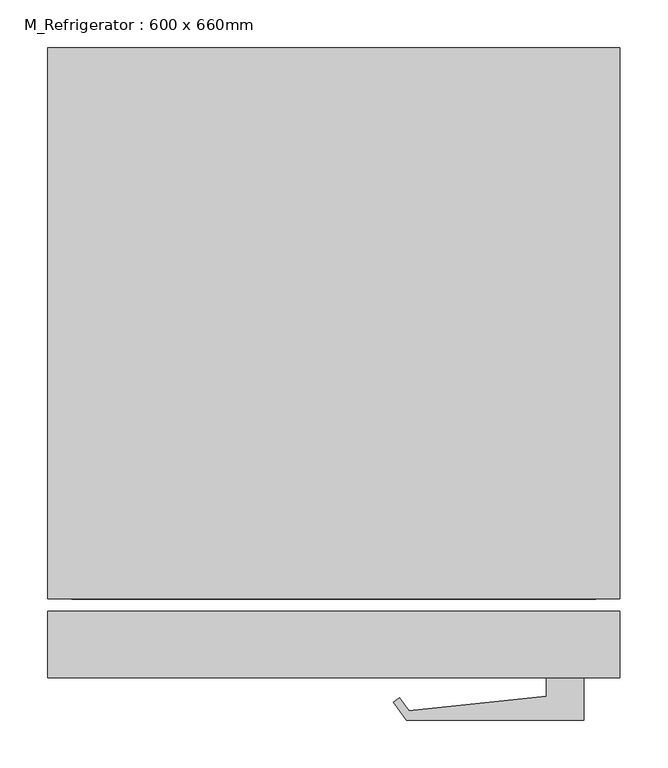
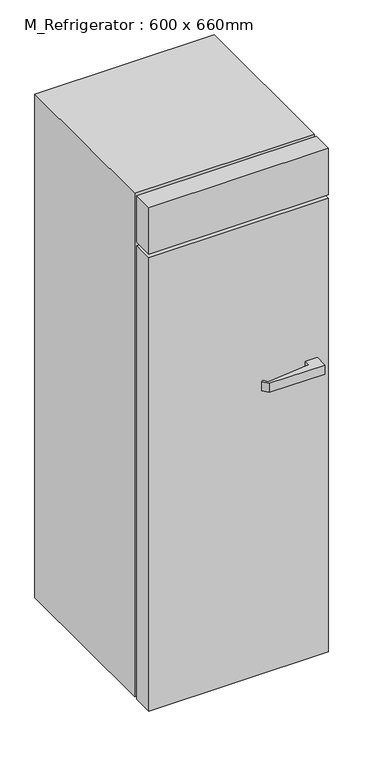
"""IFC4 building model written with IfcOpenShell, lengths in millimetres: proxy geometry, M_Refrigerator : 600 x 660mm."""

from ifc_helpers import new_model, si_unit, point, frame, frame_2d, origin, origin_with_axes, place, context, project, spatial, polyline, circle_curve, trimmed, segment, composite_curve, outline, extrude, source, transform, mapped, element, save


def m_refrigerator_600_x_660mm_a466bf94(model_context):
    return source(origin(), model_context, "Body", "SweptSolid", [
        extrude(outline(polyline([(208.0988574, -408.1036861), (22.3988574, -408.1036861), (8.7240737, -389.5368406), (15.2273026, -384.7471068), (25.1756383, -398.2543926), (168.9242419, -383.0358618), (168.9242419, -363.7849098), (208.0988574, -363.7849098), (208.0988574, -408.1036861)])), frame((0.0, 0.0, 1071.927792), z_axis=(0.0, 0.0, 1.0), x_axis=(1.0, 0.0, 0.0)), (0.0, 0.0, 1.0), 31.75),
        extrude(outline(composite_curve([segment(trimmed(circle_curve(frame_2d((-271.2511426, 220.0150902)), 25.4), [point((-296.6511426, 220.0150902))], [point((-245.8511426, 220.0150902))], False, "CARTESIAN"), True, "CONTINUOUS"), segment(trimmed(circle_curve(frame_2d((-271.2511426, 220.0150902)), 25.4), [point((-245.8511426, 220.0150902))], [point((-296.6511426, 220.0150902))], False, "CARTESIAN"), True, "CONTINUOUS")], self_intersect=False)), origin_with_axes(), (0.0, 0.0, 1.0), 50.8),
        extrude(outline(composite_curve([segment(trimmed(circle_curve(frame_2d((163.6488574, 220.0150902)), 25.4), [point((138.2488574, 220.0150902))], [point((189.0488574, 220.0150902))], False, "CARTESIAN"), True, "CONTINUOUS"), segment(trimmed(circle_curve(frame_2d((163.6488574, 220.0150902)), 25.4), [point((189.0488574, 220.0150902))], [point((138.2488574, 220.0150902))], False, "CARTESIAN"), True, "CONTINUOUS")], self_intersect=False)), origin_with_axes(), (0.0, 0.0, 1.0), 50.8),
        extrude(outline(composite_curve([segment(trimmed(circle_curve(frame_2d((-271.2511426, -236.7849098)), 25.4), [point((-296.6511426, -236.7849098))], [point((-245.8511426, -236.7849098))], False, "CARTESIAN"), True, "CONTINUOUS"), segment(trimmed(circle_curve(frame_2d((-271.2511426, -236.7849098)), 25.4), [point((-245.8511426, -236.7849098))], [point((-296.6511426, -236.7849098))], False, "CARTESIAN"), True, "CONTINUOUS")], self_intersect=False)), origin_with_axes(), (0.0, 0.0, 1.0), 50.8),
        extrude(outline(composite_curve([segment(trimmed(circle_curve(frame_2d((163.6488574, -236.7849098)), 25.4), [point((138.2488574, -236.7849098))], [point((189.0488574, -236.7849098))], False, "CARTESIAN"), True, "CONTINUOUS"), segment(trimmed(circle_curve(frame_2d((163.6488574, -236.7849098)), 25.4), [point((189.0488574, -236.7849098))], [point((138.2488574, -236.7849098))], False, "CARTESIAN"), True, "CONTINUOUS")], self_intersect=False)), origin_with_axes(), (0.0, 0.0, 1.0), 50.8),
        extrude(outline(polyline([(246.1988574, -363.7849098), (-353.8011426, -363.7849098), (-353.8011426, -293.9349098), (246.1988574, -293.9349098), (246.1988574, -363.7849098)])), frame((0.0, 0.0, 50.8), z_axis=(0.0, 0.0, 1.0), x_axis=(1.0, 0.0, 0.0)), (0.0, 0.0, 1.0), 1601.4),
        extrude(outline(polyline([(246.1988574, -363.7849098), (-353.8011426, -363.7849098), (-353.8011426, -293.9349098), (246.1988574, -293.9349098), (246.1988574, -363.7849098)])), frame((0.0, 0.0, 1664.9), z_axis=(0.0, 0.0, 1.0), x_axis=(1.0, 0.0, 0.0)), (0.0, 0.0, 1.0), 165.1),
        extrude(outline(polyline([(220.7988574, 270.8150902), (-328.4011426, 270.8150902), (-328.4011426, 296.2150902), (220.7988574, 296.2150902), (220.7988574, 270.8150902)])), frame((0.0, 0.0, 152.4), z_axis=(0.0, 0.0, 1.0), x_axis=(1.0, 0.0, 0.0)), (0.0, 0.0, 1.0), 1652.2),
        extrude(outline(polyline([(1830.0, 246.1988574), (1830.0, -353.8011426), (50.8, -353.8011426), (50.8, 246.1988574), (1830.0, 246.1988574)]), holes=[polyline([(1626.8, 220.7988574), (431.8, 220.7988574), (431.8, -328.4011426), (1626.8, -328.4011426), (1626.8, 220.7988574)])]), frame((0.0, -281.2349098, 0.0), z_axis=(0.0, 1.0, 0.0), x_axis=(0.0, 0.0, 1.0)), (0.0, 0.0, 1.0), 577.45),
    ])


if __name__ == "__main__":
    model = new_model("IFC4")
    model_context = context("Model", 3, world=origin())
    ifc_project = project(units=[si_unit("LENGTHUNIT", "METRE", prefix="MILLI")], contexts=[model_context])
    site = spatial("IfcSite", under=ifc_project)
    building = spatial("IfcBuilding", under=site)
    placement = place(None, origin())
    m_refrigerator_600_x_660mm_shape = m_refrigerator_600_x_660mm_a466bf94(model_context)
    element("IfcBuildingElementProxy", 1, Name="M_Refrigerator : 600 x 660mm", ObjectType="M_Refrigerator : 600 x 660mm", at=placement, inside=building, context=model_context, shape_type="MappedRepresentation", body=[
        mapped(m_refrigerator_600_x_660mm_shape, transform((0.0, 0.0, 0.0), x_axis=(1.0, 0.0, 0.0), y_axis=(0.0, 1.0, 0.0), z_axis=(0.0, 0.0, 1.0))),
    ])
    save(model, "model.ifc")

# Revit data of these elements
# Type "M_Refrigerator : 600 x 660mm"
#   Label = "REF."
#   Depth = 660 mm
#   Height = 1830 mm
#   Width = 600 mm
#   Material = Steel, Paint Finish, Ivory, Matte
#   Description = (empty or 0)
#   Default Elevation = 0
# Element 1 (IfcBuildingElementProxy, "M_Refrigerator : 600 x 660mm")
#   Materials on its faces: "Steel, Paint Finish, Ivory, Matte", "Steel, Chrome Plated"
# Materials
#   "Steel, Paint Finish, Ivory, Matte": class "Metal", colour RGB 247 247 239, transparency 0, Description = "Steel, paint finish, ivory, matte", Cost = 0
#   "Steel, Chrome Plated": class "Metal", colour RGB 244 244 244, transparency 0, Description = "Chromiuim plated steel", Cost = 0
